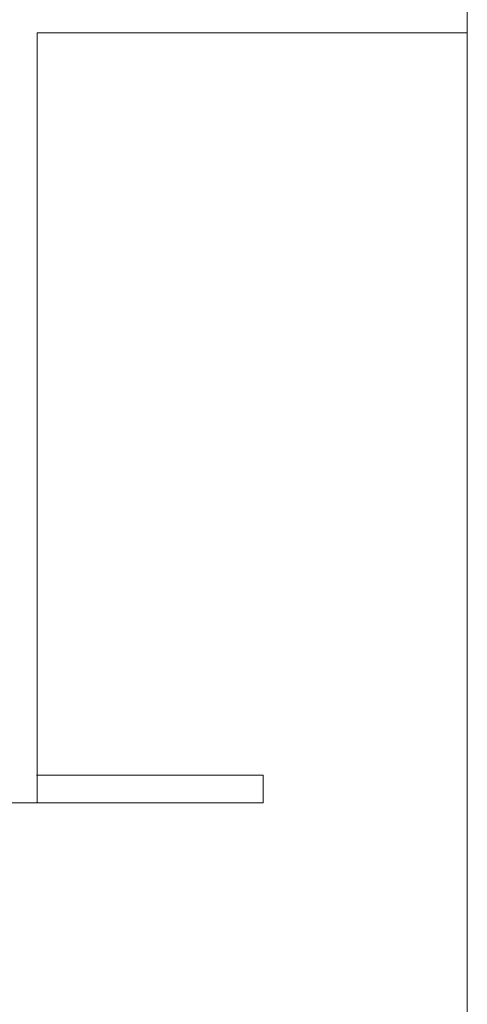
# Model space of a CAD drawing. Units: inches. Extents: x -17 to 1735, y -531 to 60.
# Tile 25 of 27: x 1734.81184 to 1734.82789, y -150.22283 to -150.18755. Entities that reach past the tile are written whole.
import ezdxf

# ---------------------------------------------------------------- set-up
doc = ezdxf.new("R2010")
doc.units = ezdxf.units.IN
doc.header["$MEASUREMENT"] = 0
doc.layers.add('A-FURN', color=242, linetype='Continuous', lineweight=18, true_color=0xcd2027)

# ---------------------------------------------------------------- blocks, each defined once
blk = doc.blocks.new('childrens_room_2')
for p, q in [((74.04826, 55.53364), (74.04826, 52.93364)), ((73.6566, 54.17714), (73.6566, 54.87789)), ((74.04826, 54.87789), (73.6566, 54.87789)), ((73.86245, 54.20212), (73.65616, 54.20212)), ((73.86245, 54.20212), (73.86245, 54.17714)), ((73.86245, 54.17714), (73.12162, 54.17714))]:
    blk.add_line(p, q)

msp = doc.modelspace()

# ---------------------------------------------------------------- block references
at = {"layer": 'A-FURN', "xscale": 0.0393700787401575, "yscale": 0.0393700787401575, "zscale": 0.0393700787401575}
msp.add_blockref('childrens_room_2', (1731.912601, -152.348565), dxfattribs=at)

doc.saveas('drawing.dxf')
